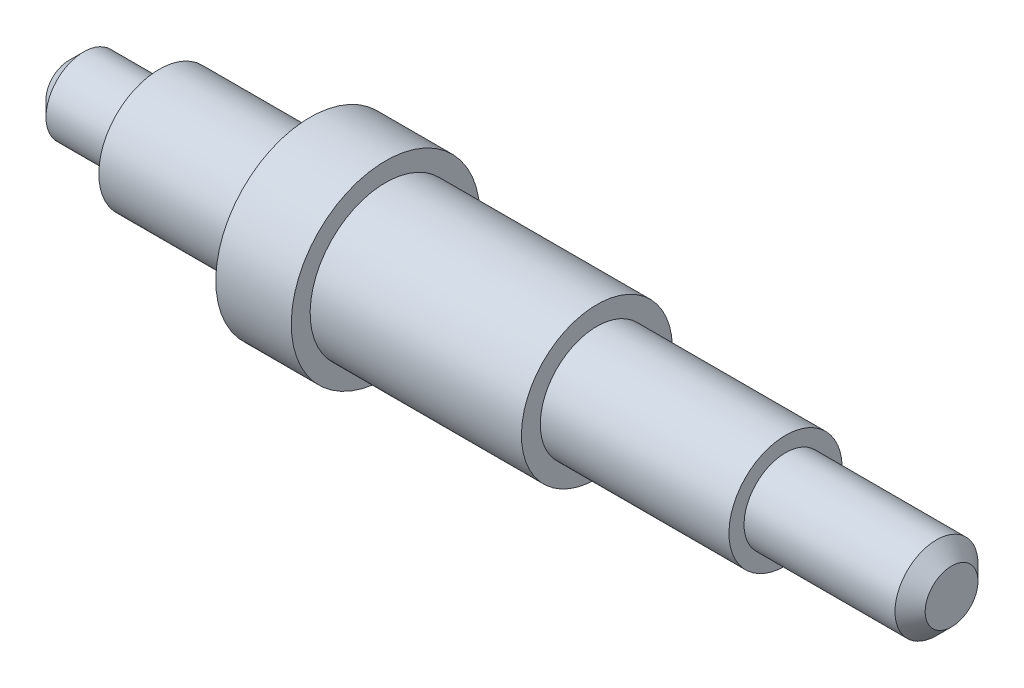
ISO-10303-21;
HEADER;
FILE_DESCRIPTION(('STEP AP214'),'2;1');
FILE_NAME('part.step','',(''),(''),'','','');
FILE_SCHEMA(('AUTOMOTIVE_DESIGN { 1 0 10303 214 1 1 1 1 }'));
ENDSEC;
DATA;
#1=APPLICATION_CONTEXT('core data for automotive mechanical design processes');
#2=APPLICATION_PROTOCOL_DEFINITION('international standard','automotive_design',2000,#1);
#3=PRODUCT_CONTEXT('',#1,'mechanical');
#4=PRODUCT('Part','Part','',(#3));
#5=PRODUCT_RELATED_PRODUCT_CATEGORY('part','',(#4));
#6=PRODUCT_DEFINITION_FORMATION('','',#4);
#7=PRODUCT_DEFINITION_CONTEXT('part definition',#1,'design');
#8=PRODUCT_DEFINITION('design','',#6,#7);
#9=PRODUCT_DEFINITION_SHAPE('','',#8);
#10=(LENGTH_UNIT() NAMED_UNIT(*) SI_UNIT(.MILLI.,.METRE.));
#11=(NAMED_UNIT(*) PLANE_ANGLE_UNIT() SI_UNIT($,.RADIAN.));
#12=(NAMED_UNIT(*) SI_UNIT($,.STERADIAN.) SOLID_ANGLE_UNIT());
#13=UNCERTAINTY_MEASURE_WITH_UNIT(LENGTH_MEASURE(1.E-05),#10,'distance_accuracy_value','');
#14=(GEOMETRIC_REPRESENTATION_CONTEXT(3) GLOBAL_UNCERTAINTY_ASSIGNED_CONTEXT((#13)) GLOBAL_UNIT_ASSIGNED_CONTEXT((#10,
#11,#12)) REPRESENTATION_CONTEXT('',''));
#15=CARTESIAN_POINT('',(0.,0.,0.));
#16=DIRECTION('',(0.,0.,1.));
#17=DIRECTION('',(1.,0.,0.));
#18=AXIS2_PLACEMENT_3D('',#15,#16,#17);
#19=CARTESIAN_POINT('',(-58.5,0.,0.));
#20=DIRECTION('',(-1.,0.,0.));
#21=DIRECTION('',(0.,-1.,0.));
#22=AXIS2_PLACEMENT_3D('',#19,#20,#21);
#23=PLANE('',#22);
#24=CARTESIAN_POINT('',(-58.5,0.,0.));
#25=DIRECTION('',(-1.,0.,0.));
#26=DIRECTION('',(0.,-1.,0.));
#27=AXIS2_PLACEMENT_3D('',#24,#25,#26);
#28=CIRCLE('',#27,3.00000000000002);
#29=CARTESIAN_POINT('',(-58.5,-3.00000000000002,0.));
#30=VERTEX_POINT('',#29);
#31=EDGE_CURVE('E54',#30,#30,#28,.T.);
#32=ORIENTED_EDGE('',*,*,#31,.T.);
#33=EDGE_LOOP('',(#32));
#34=FACE_BOUND('',#33,.T.);
#35=ADVANCED_FACE('F39',(#34),#23,.T.);
#36=CARTESIAN_POINT('',(-58.5,0.,0.));
#37=DIRECTION('',(-1.,0.,0.));
#38=DIRECTION('',(0.,-1.,0.));
#39=AXIS2_PLACEMENT_3D('',#36,#37,#38);
#40=CYLINDRICAL_SURFACE('',#39,5.);
#41=CARTESIAN_POINT('',(-56.5,0.,0.));
#42=DIRECTION('',(-1.,0.,0.));
#43=DIRECTION('',(0.,-1.,0.));
#44=AXIS2_PLACEMENT_3D('',#41,#42,#43);
#45=CIRCLE('',#44,5.);
#46=CARTESIAN_POINT('',(-56.5,-5.,0.));
#47=VERTEX_POINT('',#46);
#48=EDGE_CURVE('E51',#47,#47,#45,.F.);
#49=ORIENTED_EDGE('',*,*,#48,.T.);
#50=EDGE_LOOP('',(#49));
#51=FACE_BOUND('',#50,.T.);
#52=CARTESIAN_POINT('',(-46.5,0.,0.));
#53=DIRECTION('',(-1.,0.,0.));
#54=DIRECTION('',(0.,-1.,0.));
#55=AXIS2_PLACEMENT_3D('',#52,#53,#54);
#56=CIRCLE('',#55,5.);
#57=CARTESIAN_POINT('',(-46.5,-5.,0.));
#58=VERTEX_POINT('',#57);
#59=EDGE_CURVE('E58',#58,#58,#56,.T.);
#60=ORIENTED_EDGE('',*,*,#59,.T.);
#61=EDGE_LOOP('',(#60));
#62=FACE_BOUND('',#61,.T.);
#63=ADVANCED_FACE('F107',(#51,#62),#40,.T.);
#64=CARTESIAN_POINT('',(-46.5,-5.,0.));
#65=DIRECTION('',(-1.,0.,0.));
#66=DIRECTION('',(0.,-1.,0.));
#67=AXIS2_PLACEMENT_3D('',#64,#65,#66);
#68=PLANE('',#67);
#69=CARTESIAN_POINT('',(-46.5,0.,0.));
#70=DIRECTION('',(-1.,0.,0.));
#71=DIRECTION('',(0.,-1.,0.));
#72=AXIS2_PLACEMENT_3D('',#69,#70,#71);
#73=CIRCLE('',#72,8.);
#74=CARTESIAN_POINT('',(-46.5,-8.,0.));
#75=VERTEX_POINT('',#74);
#76=EDGE_CURVE('E62',#75,#75,#73,.T.);
#77=ORIENTED_EDGE('',*,*,#76,.T.);
#78=EDGE_LOOP('',(#77));
#79=FACE_BOUND('',#78,.T.);
#80=ORIENTED_EDGE('',*,*,#59,.F.);
#81=EDGE_LOOP('',(#80));
#82=FACE_BOUND('',#81,.T.);
#83=ADVANCED_FACE('F114',(#79,#82),#68,.T.);
#84=CARTESIAN_POINT('',(-58.5,0.,0.));
#85=DIRECTION('',(-1.,0.,0.));
#86=DIRECTION('',(0.,-1.,0.));
#87=AXIS2_PLACEMENT_3D('',#84,#85,#86);
#88=CYLINDRICAL_SURFACE('',#87,8.);
#89=CARTESIAN_POINT('',(-26.5,0.,0.));
#90=DIRECTION('',(-1.,0.,0.));
#91=DIRECTION('',(0.,-1.,0.));
#92=AXIS2_PLACEMENT_3D('',#89,#90,#91);
#93=CIRCLE('',#92,8.00000000000001);
#94=CARTESIAN_POINT('',(-26.5,-8.,0.));
#95=VERTEX_POINT('',#94);
#96=EDGE_CURVE('E67',#95,#95,#93,.T.);
#97=ORIENTED_EDGE('',*,*,#96,.T.);
#98=EDGE_LOOP('',(#97));
#99=FACE_BOUND('',#98,.T.);
#100=ORIENTED_EDGE('',*,*,#76,.F.);
#101=EDGE_LOOP('',(#100));
#102=FACE_BOUND('',#101,.T.);
#103=ADVANCED_FACE('F132',(#99,#102),#88,.T.);
#104=CARTESIAN_POINT('',(-26.5,-8.,0.));
#105=DIRECTION('',(-1.,0.,0.));
#106=DIRECTION('',(0.,-1.,0.));
#107=AXIS2_PLACEMENT_3D('',#104,#105,#106);
#108=PLANE('',#107);
#109=CARTESIAN_POINT('',(-26.5,0.,0.));
#110=DIRECTION('',(-1.,0.,0.));
#111=DIRECTION('',(0.,-1.,0.));
#112=AXIS2_PLACEMENT_3D('',#109,#110,#111);
#113=CIRCLE('',#112,12.5);
#114=CARTESIAN_POINT('',(-26.5,-12.5,0.));
#115=VERTEX_POINT('',#114);
#116=EDGE_CURVE('E69',#115,#115,#113,.T.);
#117=ORIENTED_EDGE('',*,*,#116,.T.);
#118=EDGE_LOOP('',(#117));
#119=FACE_BOUND('',#118,.T.);
#120=ORIENTED_EDGE('',*,*,#96,.F.);
#121=EDGE_LOOP('',(#120));
#122=FACE_BOUND('',#121,.T.);
#123=ADVANCED_FACE('F138',(#119,#122),#108,.T.);
#124=CARTESIAN_POINT('',(-58.5,0.,0.));
#125=DIRECTION('',(-1.,0.,0.));
#126=DIRECTION('',(0.,-1.,0.));
#127=AXIS2_PLACEMENT_3D('',#124,#125,#126);
#128=CYLINDRICAL_SURFACE('',#127,12.5);
#129=CARTESIAN_POINT('',(-16.5,0.,0.));
#130=DIRECTION('',(-1.,0.,0.));
#131=DIRECTION('',(0.,-1.,0.));
#132=AXIS2_PLACEMENT_3D('',#129,#130,#131);
#133=CIRCLE('',#132,12.5);
#134=CARTESIAN_POINT('',(-16.5,-12.5,0.));
#135=VERTEX_POINT('',#134);
#136=EDGE_CURVE('E75',#135,#135,#133,.T.);
#137=ORIENTED_EDGE('',*,*,#136,.T.);
#138=EDGE_LOOP('',(#137));
#139=FACE_BOUND('',#138,.T.);
#140=ORIENTED_EDGE('',*,*,#116,.F.);
#141=EDGE_LOOP('',(#140));
#142=FACE_BOUND('',#141,.T.);
#143=ADVANCED_FACE('F145',(#139,#142),#128,.T.);
#144=CARTESIAN_POINT('',(-16.5,-12.5,0.));
#145=DIRECTION('',(1.,0.,0.));
#146=DIRECTION('',(0.,1.,0.));
#147=AXIS2_PLACEMENT_3D('',#144,#145,#146);
#148=PLANE('',#147);
#149=CARTESIAN_POINT('',(-16.5,0.,0.));
#150=DIRECTION('',(-1.,0.,0.));
#151=DIRECTION('',(0.,-1.,0.));
#152=AXIS2_PLACEMENT_3D('',#149,#150,#151);
#153=CIRCLE('',#152,10.);
#154=CARTESIAN_POINT('',(-16.5,-10.,0.));
#155=VERTEX_POINT('',#154);
#156=EDGE_CURVE('E73',#155,#155,#153,.T.);
#157=ORIENTED_EDGE('',*,*,#156,.T.);
#158=EDGE_LOOP('',(#157));
#159=FACE_BOUND('',#158,.T.);
#160=ORIENTED_EDGE('',*,*,#136,.F.);
#161=EDGE_LOOP('',(#160));
#162=FACE_BOUND('',#161,.T.);
#163=ADVANCED_FACE('F146',(#159,#162),#148,.T.);
#164=CARTESIAN_POINT('',(-58.5,0.,0.));
#165=DIRECTION('',(-1.,0.,0.));
#166=DIRECTION('',(0.,-1.,0.));
#167=AXIS2_PLACEMENT_3D('',#164,#165,#166);
#168=CYLINDRICAL_SURFACE('',#167,10.);
#169=CARTESIAN_POINT('',(11.5,0.,0.));
#170=DIRECTION('',(-1.,0.,0.));
#171=DIRECTION('',(0.,-1.,0.));
#172=AXIS2_PLACEMENT_3D('',#169,#170,#171);
#173=CIRCLE('',#172,10.);
#174=CARTESIAN_POINT('',(11.5,-10.,0.));
#175=VERTEX_POINT('',#174);
#176=EDGE_CURVE('E77',#175,#175,#173,.T.);
#177=ORIENTED_EDGE('',*,*,#176,.T.);
#178=EDGE_LOOP('',(#177));
#179=FACE_BOUND('',#178,.T.);
#180=ORIENTED_EDGE('',*,*,#156,.F.);
#181=EDGE_LOOP('',(#180));
#182=FACE_BOUND('',#181,.T.);
#183=ADVANCED_FACE('F155',(#179,#182),#168,.T.);
#184=CARTESIAN_POINT('',(11.5,-10.,0.));
#185=DIRECTION('',(1.,0.,0.));
#186=DIRECTION('',(0.,1.,0.));
#187=AXIS2_PLACEMENT_3D('',#184,#185,#186);
#188=PLANE('',#187);
#189=CARTESIAN_POINT('',(11.5,0.,0.));
#190=DIRECTION('',(-1.,0.,0.));
#191=DIRECTION('',(0.,-1.,0.));
#192=AXIS2_PLACEMENT_3D('',#189,#190,#191);
#193=CIRCLE('',#192,7.50000000000001);
#194=CARTESIAN_POINT('',(11.5,-7.5,0.));
#195=VERTEX_POINT('',#194);
#196=EDGE_CURVE('E82',#195,#195,#193,.T.);
#197=ORIENTED_EDGE('',*,*,#196,.T.);
#198=EDGE_LOOP('',(#197));
#199=FACE_BOUND('',#198,.T.);
#200=ORIENTED_EDGE('',*,*,#176,.F.);
#201=EDGE_LOOP('',(#200));
#202=FACE_BOUND('',#201,.T.);
#203=ADVANCED_FACE('F156',(#199,#202),#188,.T.);
#204=CARTESIAN_POINT('',(-58.5,0.,0.));
#205=DIRECTION('',(-1.,0.,0.));
#206=DIRECTION('',(0.,-1.,0.));
#207=AXIS2_PLACEMENT_3D('',#204,#205,#206);
#208=CYLINDRICAL_SURFACE('',#207,7.50000000000002);
#209=CARTESIAN_POINT('',(36.5,0.,0.));
#210=DIRECTION('',(-1.,0.,0.));
#211=DIRECTION('',(0.,-1.,0.));
#212=AXIS2_PLACEMENT_3D('',#209,#210,#211);
#213=CIRCLE('',#212,7.50000000000002);
#214=CARTESIAN_POINT('',(36.5,-7.5,0.));
#215=VERTEX_POINT('',#214);
#216=EDGE_CURVE('E84',#215,#215,#213,.T.);
#217=ORIENTED_EDGE('',*,*,#216,.T.);
#218=EDGE_LOOP('',(#217));
#219=FACE_BOUND('',#218,.T.);
#220=ORIENTED_EDGE('',*,*,#196,.F.);
#221=EDGE_LOOP('',(#220));
#222=FACE_BOUND('',#221,.T.);
#223=ADVANCED_FACE('F104',(#219,#222),#208,.T.);
#224=CARTESIAN_POINT('',(36.5,-7.5,0.));
#225=DIRECTION('',(1.,0.,0.));
#226=DIRECTION('',(0.,1.,0.));
#227=AXIS2_PLACEMENT_3D('',#224,#225,#226);
#228=PLANE('',#227);
#229=CARTESIAN_POINT('',(36.5,0.,0.));
#230=DIRECTION('',(-1.,0.,0.));
#231=DIRECTION('',(0.,-1.,0.));
#232=AXIS2_PLACEMENT_3D('',#229,#230,#231);
#233=CIRCLE('',#232,5.50000000000002);
#234=CARTESIAN_POINT('',(36.5,-5.5,0.));
#235=VERTEX_POINT('',#234);
#236=EDGE_CURVE('E87',#235,#235,#233,.T.);
#237=ORIENTED_EDGE('',*,*,#236,.T.);
#238=EDGE_LOOP('',(#237));
#239=FACE_BOUND('',#238,.T.);
#240=ORIENTED_EDGE('',*,*,#216,.F.);
#241=EDGE_LOOP('',(#240));
#242=FACE_BOUND('',#241,.T.);
#243=ADVANCED_FACE('F93',(#239,#242),#228,.T.);
#244=CARTESIAN_POINT('',(-58.5,0.,0.));
#245=DIRECTION('',(-1.,0.,0.));
#246=DIRECTION('',(0.,-1.,0.));
#247=AXIS2_PLACEMENT_3D('',#244,#245,#246);
#248=CYLINDRICAL_SURFACE('',#247,5.50000000000002);
#249=CARTESIAN_POINT('',(56.5,0.,0.));
#250=DIRECTION('',(1.,0.,0.));
#251=DIRECTION('',(0.,1.,0.));
#252=AXIS2_PLACEMENT_3D('',#249,#250,#251);
#253=CIRCLE('',#252,5.50000000000002);
#254=CARTESIAN_POINT('',(56.5,5.50000000000004,0.));
#255=VERTEX_POINT('',#254);
#256=EDGE_CURVE('E50',#255,#255,#253,.F.);
#257=ORIENTED_EDGE('',*,*,#256,.T.);
#258=EDGE_LOOP('',(#257));
#259=FACE_BOUND('',#258,.T.);
#260=ORIENTED_EDGE('',*,*,#236,.F.);
#261=EDGE_LOOP('',(#260));
#262=FACE_BOUND('',#261,.T.);
#263=ADVANCED_FACE('F94',(#259,#262),#248,.T.);
#264=CARTESIAN_POINT('',(58.5,-5.5,0.));
#265=DIRECTION('',(1.,0.,0.));
#266=DIRECTION('',(0.,1.,0.));
#267=AXIS2_PLACEMENT_3D('',#264,#265,#266);
#268=PLANE('',#267);
#269=CARTESIAN_POINT('',(58.5,0.,0.));
#270=DIRECTION('',(1.,0.,0.));
#271=DIRECTION('',(0.,1.,0.));
#272=AXIS2_PLACEMENT_3D('',#269,#270,#271);
#273=CIRCLE('',#272,3.49999999999999);
#274=CARTESIAN_POINT('',(58.5,3.50000000000001,0.));
#275=VERTEX_POINT('',#274);
#276=EDGE_CURVE('E10',#275,#275,#273,.T.);
#277=ORIENTED_EDGE('',*,*,#276,.T.);
#278=EDGE_LOOP('',(#277));
#279=FACE_BOUND('',#278,.T.);
#280=ADVANCED_FACE('F96',(#279),#268,.T.);
#281=CARTESIAN_POINT('',(-58.5,0.,0.));
#282=DIRECTION('',(1.,0.,0.));
#283=DIRECTION('',(0.,1.,0.));
#284=AXIS2_PLACEMENT_3D('',#281,#282,#283);
#285=CONICAL_SURFACE('',#284,3.00000000000002,0.785398163397441);
#286=ORIENTED_EDGE('',*,*,#48,.F.);
#287=EDGE_LOOP('',(#286));
#288=FACE_BOUND('',#287,.T.);
#289=ORIENTED_EDGE('',*,*,#31,.F.);
#290=EDGE_LOOP('',(#289));
#291=FACE_BOUND('',#290,.T.);
#292=ADVANCED_FACE('F105',(#288,#291),#285,.T.);
#293=CARTESIAN_POINT('',(56.5,0.,0.));
#294=DIRECTION('',(-1.,0.,0.));
#295=DIRECTION('',(0.,-1.,0.));
#296=AXIS2_PLACEMENT_3D('',#293,#294,#295);
#297=CONICAL_SURFACE('',#296,5.50000000000002,0.785398163397452);
#298=ORIENTED_EDGE('',*,*,#276,.F.);
#299=EDGE_LOOP('',(#298));
#300=FACE_BOUND('',#299,.T.);
#301=ORIENTED_EDGE('',*,*,#256,.F.);
#302=EDGE_LOOP('',(#301));
#303=FACE_BOUND('',#302,.T.);
#304=ADVANCED_FACE('F45',(#300,#303),#297,.T.);
#305=CLOSED_SHELL('',(#35,#63,#83,#103,#123,#143,#163,#183,#203,#223,#243,#263,#280,#292,#304));
#306=MANIFOLD_SOLID_BREP('B2',#305);
#307=ADVANCED_BREP_SHAPE_REPRESENTATION('',(#18,#306),#14);
#308=SHAPE_DEFINITION_REPRESENTATION(#9,#307);
ENDSEC;
END-ISO-10303-21;
